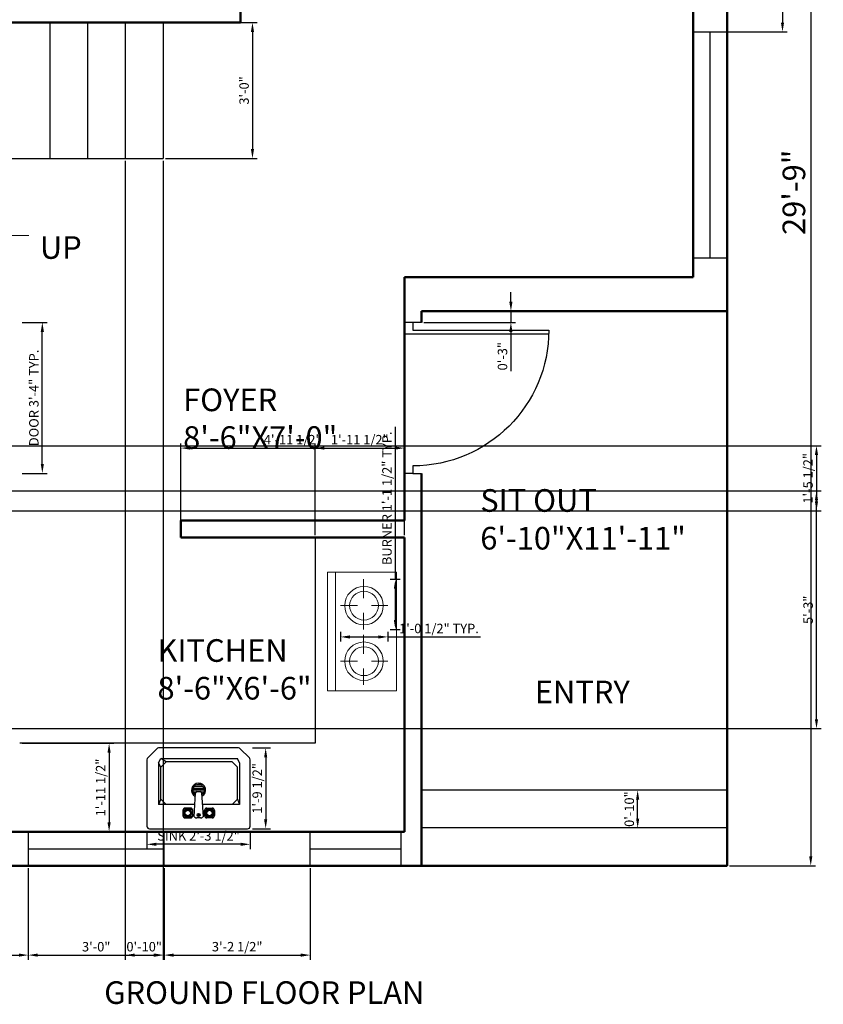
# Model space of a CAD drawing. Units: inches. Extents: x 3242 to 3618, y 1365 to 1814.
# Tile 3 of 6: x 3405 to 3618, y 1365 to 1626. Entities that reach past the tile are written whole.
import ezdxf

# ---------------------------------------------------------------- set-up
doc = ezdxf.new("R2010")
doc.units = ezdxf.units.IN
for name, color, linetype, lineweight in [('A-ANNO-DIMS', 2, 'Continuous', 18), ('A-ANNO-SYMB', 7, 'Continuous', 18), ('A-ANNO-TEXT', 7, 'Continuous', 25), ('A-AREA-IDEN', 7, 'Continuous', 25), ('A-DOOR', 4, 'Continuous', 25), ('A-EQPM', 8, 'Continuous', 18), ('A-FLOR-CASE', 8, 'Continuous', 25), ('A-FLOR-FIXT', 8, 'Continuous', 25), ('A-FLOR-STRS', 7, 'Continuous', 25), ('A-GLAZ', 5, 'Continuous', 25), ('A-WALL', 7, 'Continuous', 50)]:
    doc.layers.add(name, color=color, linetype=linetype, lineweight=lineweight)
doc.styles.get("Standard").update_dxf_attribs({"font": 'arial.ttf'})
doc.dimstyles.new('ISO-25', dxfattribs={"dimtxt": 2.5, "dimasz": 2.5, "dimexe": 1.25, "dimexo": 0.625, "dimtad": 1, "dimdec": 0, "dimlunit": 3, "dimtxsty": 'Standard', "dimcen": 2.5, "dimadec": 0, "dimazin": 0, "dimtfac": 1, "dimtdec": 0, "dimtmove": 0, "dimatfit": 3, "dimfxl": 1, "dimarcsym": 0})

# ---------------------------------------------------------------- blocks, each defined once
blk = doc.blocks.new('A$C4CB854FF')
for p, q in [((0.4725, 0.38), (0.0125, 0.38)), ((0, 0.3675), (0, 0.0552)), ((0.1787, 0.329), (0.2034, 0.329)), ((0.2337, 0.329), (0.2502, 0.329)), ((0.3052, 0.329), (0.2804, 0.329)), ((0.485, 0.0552), (0.485, 0.3675)), ((0.1677, 0.2932), (0.1677, 0.318)), ((0.1745, 0.2919), (0.1745, 0.3194)), ((0.1773, 0.3221), (0.2048, 0.3221)), ((0.2048, 0.2891), (0.1773, 0.2891)), ((0.2034, 0.2822), (0.1787, 0.2822)), ((0.2075, 0.3194), (0.2075, 0.2919)), ((0.2144, 0.318), (0.2144, 0.2932)), ((0.2279, 0.2104), (0.2213, 0.3235)), ((0.2625, 0.3235), (0.256, 0.2104)), ((0.2694, 0.318), (0.2694, 0.2932)), ((0.2763, 0.3194), (0.2763, 0.2919)), ((0.3065, 0.3221), (0.279, 0.3221)), ((0.279, 0.2891), (0.3065, 0.2891)), ((0.2804, 0.2822), (0.3052, 0.2822)), ((0.3093, 0.2919), (0.3093, 0.3194)), ((0.3162, 0.2932), (0.3162, 0.318)), ((0.05, 0.265), (0.2247, 0.265)), ((0.06, 0.24), (0.05, 0.265)), ((0.05, 0.07), (0.05, 0.265)), ((0.085, 0.265), (0.06, 0.24)), ((0.06, 0.24), (0.06, 0.09)), ((0.2591, 0.265), (0.43, 0.265)), ((0.395, 0.265), (0.42, 0.24)), ((0.42, 0.24), (0.43, 0.265)), ((0.42, 0.24), (0.42, 0.09)), ((0.43, 0.07), (0.43, 0.265)), ((0.2152, 0.1984), (0.2694, 0.1984)), ((0.2297, 0.2066), (0.2165, 0.2066)), ((0.2681, 0.1901), (0.2165, 0.1901)), ((0.2272, 0.2149), (0.2208, 0.2149)), ((0.2505, 0.2052), (0.2334, 0.2052)), ((0.2681, 0.2066), (0.2541, 0.2066)), ((0.2638, 0.2149), (0.2566, 0.2149)), ((0.2638, 0.1819), (0.2208, 0.1819)), ((0.2533, 0.1736), (0.2313, 0.1736)), ((0.0037, 0.0463), (0.0463, 0.0037)), ((0.05, 0.07), (0.06, 0.05)), ((0.06, 0.09), (0.085, 0.065)), ((0.42, 0.05), (0.06, 0.05)), ((0.085, 0.065), (0.395, 0.065)), ((0.42, 0.09), (0.395, 0.065)), ((0.395, 0.065), (0.42, 0.05)), ((0.42, 0.09), (0.43, 0.07)), ((0.43, 0.07), (0.42, 0.05)), ((0.4387, 0.0037), (0.4813, 0.0463)), ((0.0552, 0), (0.4298, 0))]:
    blk.add_line(p, q)
for centre, radius in [((0.191, 0.3056), 0.0165), ((0.191, 0.3056), 0.0127), ((0.2419, 0.3152), 0.00688), ((0.2419, 0.3152), 0.00344), ((0.2928, 0.3056), 0.0165), ((0.2928, 0.3056), 0.0127)]:
    blk.add_circle(centre, radius)
for centre, radius, start, end in [((0.0125, 0.3675), 0.0125, 90, 180), ((0.4725, 0.3675), 0.0125, 0, 90), ((0.1787, 0.318), 0.011, 90, 180), ((0.2034, 0.318), 0.011, 0, 90), ((0.2329, 0.314), 0.015, 87.1975, 140.7274), ((0.2509, 0.314), 0.015, 39.2726, 92.8025), ((0.2804, 0.318), 0.011, 90, 180), ((0.3052, 0.318), 0.011, 0, 90), ((0.1787, 0.2932), 0.011, 180, 270), ((0.1773, 0.3194), 0.00275, 90, 180), ((0.1773, 0.2919), 0.00275, 180, 270), ((0.2034, 0.2932), 0.011, 270, 0), ((0.2048, 0.3194), 0.00275, 360, 90), ((0.2048, 0.2919), 0.00275, 270, 0), ((0.2804, 0.2932), 0.011, 180, 270), ((0.279, 0.3194), 0.00275, 90, 180), ((0.279, 0.2919), 0.00275, 180, 270), ((0.3052, 0.2932), 0.011, 270, 360), ((0.3065, 0.3194), 0.00275, 360, 90), ((0.3065, 0.2919), 0.00275, 270, 0), ((0.2423, 0.1984), 0.033, 118.6883, 62.8686), ((0.2423, 0.1984), 0.0271, 124.7758, 57.2247), ((0.2334, 0.2107), 0.0055, 183.3274, 270), ((0.2505, 0.2107), 0.0055, 270, 356.6726), ((0.0125, 0.0552), 0.0125, 180, 225), ((0.4725, 0.0552), 0.0125, 315, 0), ((0.0552, 0.0125), 0.0125, 225, 270), ((0.4298, 0.0125), 0.0125, 270, 315)]:
    blk.add_arc(centre, radius, start, end)
blk = doc.blocks.new('*D4')
at = {"layer": 'A-ANNO-DIMS', "color": 0, "lineweight": -2, "transparency": 16777216}
for p, q in [((3593.11, 1758.66), (3615.91, 1758.66)), ((3614.66, 1756.16), (3614.66, 1404.16)), ((3593.11, 1401.66), (3615.91, 1401.66))]:
    blk.add_line(p, q, dxfattribs=at)
at = {"layer": 'A-ANNO-DIMS', "color": 0, "transparency": 16777216}
for points in [[(3614.24, 1756.16), (3615.08, 1756.16), (3614.66, 1758.66)], [(3614.24, 1404.16), (3615.08, 1404.16), (3614.66, 1401.66)]]:
    blk.add_solid(points, dxfattribs=at)
at = {"layer": 'Defpoints', "color": 0, "transparency": 16777216}
for p in [(3592.48, 1758.66), (3592.48, 1401.66), (3614.66, 1401.66)]:
    blk.add_point(p, dxfattribs=at)
at = {"layer": 'A-ANNO-DIMS', "color": 0, "transparency": 16777216, "insert": (3610.97, 1580.16), "char_height": 6, "attachment_point": 5, "rotation": 90}
blk.add_mtext('29\'-9"', dxfattribs=at)
blk = doc.blocks.new('DOOR-SWING-36IN')
for p, q in [((33.75, 40), (38.25, 40)), ((36, 40), (36, 38)), ((36, 38), (0, 38)), ((38.25, 37), (0, 37)), ((36, 0), (33.75, 0)), ((36, 2), (36, 0)), ((36, 0), (38.25, 0))]:
    blk.add_line(p, q)
blk.add_arc((36, 38), 36, 180, 270)
blk = doc.blocks.new('WINDOW-24IN')
for p, q in [((0, 9), (24, 9)), ((0, 0), (0, 9)), ((24, 9), (24, 0)), ((0, 4.5), (24, 4.5)), ((24, 0), (0, 0))]:
    blk.add_line(p, q)
blk = doc.blocks.new('WINDOW-60IN')
for p, q in [((0, 9), (60, 9)), ((0, 0), (0, 9)), ((60, 9), (60, 0)), ((0, 4.5), (60, 4.5)), ((60, 0), (0, 0))]:
    blk.add_line(p, q)
blk = doc.blocks.new('COOKTOP-BURNER')
at = {"ltscale": 120}
for p, q in [((6.09, 13.3), (6.09, 8.26)), ((0, 6.34), (4.54, 6.34)), ((8.26, 6.34), (12.57, 6.34)), ((6.09, 4.41), (6.09, 0))]:
    blk.add_line(p, q, dxfattribs=at)
for radius in [5.11, 3.82]:
    blk.add_circle((6.23, 6.3), radius, dxfattribs=at)
blk = doc.blocks.new('*D17')
at = {"layer": 'A-ANNO-DIMS', "color": 0, "lineweight": -2, "transparency": 16777216}
for p, q in [((3405.61, 1545.66), (3412.23, 1545.66)), ((3410.98, 1508.16), (3410.98, 1543.16)), ((3405.61, 1505.66), (3412.23, 1505.66))]:
    blk.add_line(p, q, dxfattribs=at)
at = {"layer": 'A-ANNO-DIMS', "color": 0, "transparency": 16777216}
for points in [[(3410.56, 1543.16), (3411.4, 1543.16), (3410.98, 1545.66)], [(3410.56, 1508.16), (3411.4, 1508.16), (3410.98, 1505.66)]]:
    blk.add_solid(points, dxfattribs=at)
at = {"layer": 'Defpoints', "color": 0, "transparency": 16777216}
for p in [(3404.98, 1545.66), (3410.98, 1545.66), (3404.98, 1505.66)]:
    blk.add_point(p, dxfattribs=at)
at = {"layer": 'A-ANNO-DIMS', "color": 0, "transparency": 16777216, "insert": (3409.06, 1525.66), "char_height": 2.5, "attachment_point": 5, "rotation": 90}
blk.add_mtext('DOOR 3\'-4" TYP.', dxfattribs=at)
blk = doc.blocks.new('*D25')
at = {"layer": 'A-ANNO-DIMS', "color": 0, "lineweight": -2, "transparency": 16777216}
for p, q in [((3438.7, 1410.81), (3438.7, 1406.08)), ((3466.07, 1410.81), (3466.07, 1406.08)), ((3463.57, 1407.33), (3441.2, 1407.33))]:
    blk.add_line(p, q, dxfattribs=at)
at = {"layer": 'A-ANNO-DIMS', "color": 0, "transparency": 16777216}
for points in [[(3441.2, 1407.75), (3441.2, 1406.91), (3438.7, 1407.33)], [(3463.57, 1407.75), (3463.57, 1406.91), (3466.07, 1407.33)]]:
    blk.add_solid(points, dxfattribs=at)
at = {"layer": 'Defpoints', "color": 0, "transparency": 16777216}
for p in [(3438.7, 1411.44), (3466.07, 1411.44), (3438.7, 1407.33)]:
    blk.add_point(p, dxfattribs=at)
at = {"layer": 'A-ANNO-DIMS', "color": 0, "transparency": 16777216, "insert": (3452.38, 1409.25), "char_height": 2.5, "attachment_point": 5}
blk.add_mtext('SINK 2\'-3 1/2"', dxfattribs=at)
blk = doc.blocks.new('*D26')
at = {"layer": 'A-ANNO-DIMS', "color": 0, "lineweight": -2, "transparency": 16777216}
for p, q in [((3466.69, 1432.88), (3471.43, 1432.88)), ((3470.18, 1430.38), (3470.18, 1413.94)), ((3466.69, 1411.44), (3471.43, 1411.44))]:
    blk.add_line(p, q, dxfattribs=at)
at = {"layer": 'A-ANNO-DIMS', "color": 0, "transparency": 16777216}
for points in [[(3469.76, 1430.38), (3470.59, 1430.38), (3470.18, 1432.88)], [(3469.76, 1413.94), (3470.59, 1413.94), (3470.18, 1411.44)]]:
    blk.add_solid(points, dxfattribs=at)
at = {"layer": 'Defpoints', "color": 0, "transparency": 16777216}
for p in [(3466.07, 1432.88), (3466.07, 1411.44), (3470.18, 1411.44)]:
    blk.add_point(p, dxfattribs=at)
at = {"layer": 'A-ANNO-DIMS', "color": 0, "transparency": 16777216, "insert": (3468.26, 1422.16), "char_height": 2.5, "attachment_point": 5, "rotation": 90}
blk.add_mtext('1\'-9 1/2"', dxfattribs=at)
blk = doc.blocks.new('*D27')
at = {"layer": 'A-ANNO-DIMS', "color": 0, "lineweight": -2, "transparency": 16777216}
for p, q in [((3504.57, 1477.59), (3504.57, 1518.01)), ((3503.2, 1477.59), (3505.82, 1477.59)), ((3504.57, 1466.79), (3504.57, 1475.09)), ((3503.2, 1464.29), (3505.82, 1464.29))]:
    blk.add_line(p, q, dxfattribs=at)
at = {"layer": 'A-ANNO-DIMS', "color": 0, "transparency": 16777216}
for points in [[(3504.15, 1475.09), (3504.99, 1475.09), (3504.57, 1477.59)], [(3504.15, 1466.79), (3504.99, 1466.79), (3504.57, 1464.29)]]:
    blk.add_solid(points, dxfattribs=at)
at = {"layer": 'Defpoints', "color": 0, "transparency": 16777216}
for p in [(3502.57, 1477.59), (3504.57, 1477.59), (3502.57, 1464.29)]:
    blk.add_point(p, dxfattribs=at)
at = {"layer": 'A-ANNO-DIMS', "color": 0, "transparency": 16777216, "insert": (3502.65, 1499.05), "char_height": 2.5, "attachment_point": 5, "rotation": 90}
blk.add_mtext('BURNER 1\'-1 1/2" TYP.', dxfattribs=at)
blk = doc.blocks.new('*D28')
at = {"layer": 'A-ANNO-DIMS', "color": 0, "lineweight": -2, "transparency": 16777216}
for p, q in [((3490.01, 1463.67), (3490.01, 1461.05)), ((3492.51, 1462.3), (3500.07, 1462.3)), ((3502.57, 1463.67), (3502.57, 1461.05)), ((3502.57, 1462.3), (3527.15, 1462.3))]:
    blk.add_line(p, q, dxfattribs=at)
at = {"layer": 'A-ANNO-DIMS', "color": 0, "transparency": 16777216}
for points in [[(3492.51, 1462.71), (3492.51, 1461.88), (3490.01, 1462.3)], [(3500.07, 1462.71), (3500.07, 1461.88), (3502.57, 1462.3)]]:
    blk.add_solid(points, dxfattribs=at)
at = {"layer": 'Defpoints', "color": 0, "transparency": 16777216}
for p in [(3490.01, 1464.29), (3502.57, 1464.29), (3502.57, 1462.3)]:
    blk.add_point(p, dxfattribs=at)
at = {"layer": 'A-ANNO-DIMS', "color": 0, "transparency": 16777216, "insert": (3516.11, 1464.22), "char_height": 2.5, "attachment_point": 5}
blk.add_mtext('1\'-0 1/2" TYP.', dxfattribs=at)
blk = doc.blocks.new('*D36')
at = {"layer": 'A-ANNO-DIMS', "color": 0, "lineweight": -2, "transparency": 16777216}
for p, q in [((3584.11, 1670.23), (3608.43, 1670.23)), ((3607.18, 1667.73), (3607.18, 1625.17)), ((3584.11, 1622.67), (3608.43, 1622.67))]:
    blk.add_line(p, q, dxfattribs=at)
at = {"layer": 'A-ANNO-DIMS', "color": 0, "transparency": 16777216}
for points in [[(3606.76, 1667.73), (3607.6, 1667.73), (3607.18, 1670.23)], [(3606.76, 1625.17), (3607.6, 1625.17), (3607.18, 1622.67)]]:
    blk.add_solid(points, dxfattribs=at)
at = {"layer": 'Defpoints', "color": 0, "transparency": 16777216}
for p in [(3583.48, 1670.23), (3583.48, 1622.67), (3607.18, 1622.67)]:
    blk.add_point(p, dxfattribs=at)
at = {"layer": 'A-ANNO-DIMS', "color": 0, "transparency": 16777216, "insert": (3605.26, 1646.45), "char_height": 2.5, "attachment_point": 5, "rotation": 90}
blk.add_mtext('3\'-11 1/2"', dxfattribs=at)
blk = doc.blocks.new('*D40')
at = {"layer": 'A-ANNO-DIMS', "color": 0, "lineweight": -2, "transparency": 16777216}
for p, q in [((3375.35, 1401.03), (3375.35, 1376.71)), ((3407.26, 1401.03), (3407.26, 1376.71)), ((3377.85, 1377.96), (3404.76, 1377.96))]:
    blk.add_line(p, q, dxfattribs=at)
at = {"layer": 'A-ANNO-DIMS', "color": 0, "transparency": 16777216}
for points in [[(3377.85, 1378.37), (3377.85, 1377.54), (3375.35, 1377.96)], [(3404.76, 1378.37), (3404.76, 1377.54), (3407.26, 1377.96)]]:
    blk.add_solid(points, dxfattribs=at)
at = {"layer": 'Defpoints', "color": 0, "transparency": 16777216}
for p in [(3375.35, 1401.66), (3407.26, 1401.66), (3407.26, 1377.96)]:
    blk.add_point(p, dxfattribs=at)
at = {"layer": 'A-ANNO-DIMS', "color": 0, "transparency": 16777216, "insert": (3391.3, 1379.86), "char_height": 2.5, "attachment_point": 5}
blk.add_mtext('2\'-8"', dxfattribs=at)
blk = doc.blocks.new('*D41')
at = {"layer": 'A-ANNO-DIMS', "color": 0, "lineweight": -2, "transparency": 16777216}
for p, q in [((3407.26, 1401.03), (3407.26, 1376.71)), ((3443.26, 1401.03), (3443.26, 1376.71)), ((3409.76, 1377.96), (3440.76, 1377.96))]:
    blk.add_line(p, q, dxfattribs=at)
at = {"layer": 'A-ANNO-DIMS', "color": 0, "transparency": 16777216}
for points in [[(3409.76, 1378.37), (3409.76, 1377.54), (3407.26, 1377.96)], [(3440.76, 1378.37), (3440.76, 1377.54), (3443.26, 1377.96)]]:
    blk.add_solid(points, dxfattribs=at)
at = {"layer": 'Defpoints', "color": 0, "transparency": 16777216}
for p in [(3407.26, 1401.66), (3443.26, 1401.66), (3443.26, 1377.96)]:
    blk.add_point(p, dxfattribs=at)
at = {"layer": 'A-ANNO-DIMS', "color": 0, "transparency": 16777216, "insert": (3425.26, 1379.86), "char_height": 2.5, "attachment_point": 5}
blk.add_mtext('3\'-0"', dxfattribs=at)
blk = doc.blocks.new('*D42')
at = {"layer": 'A-ANNO-DIMS', "color": 0, "lineweight": -2, "transparency": 16777216}
for p, q in [((3443.26, 1401.03), (3443.26, 1376.71)), ((3482, 1401.03), (3482, 1376.71)), ((3445.76, 1377.96), (3479.5, 1377.96))]:
    blk.add_line(p, q, dxfattribs=at)
at = {"layer": 'A-ANNO-DIMS', "color": 0, "transparency": 16777216}
for points in [[(3445.76, 1378.37), (3445.76, 1377.54), (3443.26, 1377.96)], [(3479.5, 1378.37), (3479.5, 1377.54), (3482, 1377.96)]]:
    blk.add_solid(points, dxfattribs=at)
at = {"layer": 'Defpoints', "color": 0, "transparency": 16777216}
for p in [(3443.26, 1401.66), (3482, 1401.66), (3482, 1377.96)]:
    blk.add_point(p, dxfattribs=at)
at = {"layer": 'A-ANNO-DIMS', "color": 0, "transparency": 16777216, "insert": (3462.63, 1379.87), "char_height": 2.5, "attachment_point": 5}
blk.add_mtext('3\'-2 1/2"', dxfattribs=at)
blk = doc.blocks.new('*D43')
at = {"layer": 'A-ANNO-DIMS', "color": 0, "lineweight": -2, "transparency": 16777216}
for p, q in [((3432.98, 1588.53), (3432.98, 1376.71)), ((3442.98, 1588.53), (3442.98, 1376.71)), ((3435.48, 1377.96), (3440.48, 1377.96))]:
    blk.add_line(p, q, dxfattribs=at)
at = {"layer": 'A-ANNO-DIMS', "color": 0, "transparency": 16777216}
for points in [[(3435.48, 1378.37), (3435.48, 1377.54), (3432.98, 1377.96)], [(3440.48, 1378.37), (3440.48, 1377.54), (3442.98, 1377.96)]]:
    blk.add_solid(points, dxfattribs=at)
at = {"layer": 'Defpoints', "color": 0, "transparency": 16777216}
for p in [(3432.98, 1589.16), (3442.98, 1589.16), (3442.98, 1377.96)]:
    blk.add_point(p, dxfattribs=at)
at = {"layer": 'A-ANNO-DIMS', "color": 0, "transparency": 16777216, "insert": (3437.98, 1379.86), "char_height": 2.5, "attachment_point": 5}
blk.add_mtext('0\'-10"', dxfattribs=at)
blk = doc.blocks.new('*D44')
at = {"layer": 'A-ANNO-DIMS', "color": 0, "lineweight": -2, "transparency": 16777216}
for p, q in [((3443.61, 1625.16), (3467.93, 1625.16)), ((3466.68, 1622.66), (3466.68, 1591.66)), ((3443.61, 1589.16), (3467.93, 1589.16))]:
    blk.add_line(p, q, dxfattribs=at)
at = {"layer": 'A-ANNO-DIMS', "color": 0, "transparency": 16777216}
for points in [[(3466.26, 1622.66), (3467.1, 1622.66), (3466.68, 1625.16)], [(3466.26, 1591.66), (3467.1, 1591.66), (3466.68, 1589.16)]]:
    blk.add_solid(points, dxfattribs=at)
at = {"layer": 'Defpoints', "color": 0, "transparency": 16777216}
for p in [(3442.98, 1625.16), (3442.98, 1589.16), (3466.68, 1589.16)]:
    blk.add_point(p, dxfattribs=at)
at = {"layer": 'A-ANNO-DIMS', "color": 0, "transparency": 16777216, "insert": (3464.78, 1607.16), "char_height": 2.5, "attachment_point": 5, "rotation": 90}
blk.add_mtext('3\'-0"', dxfattribs=at)
blk = doc.blocks.new('*D45')
at = {"layer": 'A-ANNO-DIMS', "color": 0, "lineweight": -2, "transparency": 16777216}
for p, q in [((3405.61, 1434.12), (3429.93, 1434.12)), ((3428.68, 1431.62), (3428.68, 1413.16)), ((3405.61, 1410.66), (3429.93, 1410.66))]:
    blk.add_line(p, q, dxfattribs=at)
at = {"layer": 'A-ANNO-DIMS', "color": 0, "transparency": 16777216}
for points in [[(3428.26, 1431.62), (3429.1, 1431.62), (3428.68, 1434.12)], [(3428.26, 1413.16), (3429.1, 1413.16), (3428.68, 1410.66)]]:
    blk.add_solid(points, dxfattribs=at)
at = {"layer": 'Defpoints', "color": 0, "transparency": 16777216}
for p in [(3404.98, 1434.12), (3404.98, 1410.66), (3428.68, 1410.66)]:
    blk.add_point(p, dxfattribs=at)
at = {"layer": 'A-ANNO-DIMS', "color": 0, "transparency": 16777216, "insert": (3426.76, 1422.39), "char_height": 2.5, "attachment_point": 5, "rotation": 90}
blk.add_mtext('1\'-11 1/2"', dxfattribs=at)
blk = doc.blocks.new('*D46')
at = {"layer": 'A-ANNO-DIMS', "color": 0, "lineweight": -2, "transparency": 16777216}
for p, q in [((3483.26, 1489.28), (3483.26, 1513.61)), ((3485.76, 1512.36), (3504.48, 1512.36)), ((3506.98, 1489.28), (3506.98, 1513.61))]:
    blk.add_line(p, q, dxfattribs=at)
at = {"layer": 'A-ANNO-DIMS', "color": 0, "transparency": 16777216}
for points in [[(3485.76, 1512.77), (3485.76, 1511.94), (3483.26, 1512.36)], [(3504.48, 1512.77), (3504.48, 1511.94), (3506.98, 1512.36)]]:
    blk.add_solid(points, dxfattribs=at)
at = {"layer": 'Defpoints', "color": 0, "transparency": 16777216}
for p in [(3506.98, 1512.36), (3483.26, 1488.66), (3506.98, 1488.66)]:
    blk.add_point(p, dxfattribs=at)
at = {"layer": 'A-ANNO-DIMS', "color": 0, "transparency": 16777216, "insert": (3495.12, 1514.27), "char_height": 2.5, "attachment_point": 5}
blk.add_mtext('1\'-11 1/2"', dxfattribs=at)
blk = doc.blocks.new('*D54')
at = {"layer": 'A-ANNO-DIMS', "color": 0, "lineweight": -2, "transparency": 16777216}
for p, q in [((3362.21, 1500.99), (3617.43, 1500.99)), ((3616.18, 1440.49), (3616.18, 1498.49)), ((3362.21, 1437.99), (3617.43, 1437.99))]:
    blk.add_line(p, q, dxfattribs=at)
at = {"layer": 'A-ANNO-DIMS', "color": 0, "transparency": 16777216}
for points in [[(3615.76, 1498.49), (3616.6, 1498.49), (3616.18, 1500.99)], [(3615.76, 1440.49), (3616.6, 1440.49), (3616.18, 1437.99)]]:
    blk.add_solid(points, dxfattribs=at)
at = {"layer": 'Defpoints', "color": 0, "transparency": 16777216}
for p in [(3361.59, 1500.99), (3616.18, 1500.99), (3361.59, 1437.99)]:
    blk.add_point(p, dxfattribs=at)
at = {"layer": 'A-ANNO-DIMS', "color": 0, "transparency": 16777216, "insert": (3614.28, 1469.49), "char_height": 2.5, "attachment_point": 5, "rotation": 90}
blk.add_mtext('5\'-3"', dxfattribs=at)
blk = doc.blocks.new('*D55')
at = {"layer": 'A-ANNO-DIMS', "color": 0, "lineweight": -2, "transparency": 16777216}
for p, q in [((3303.13, 1513), (3617.43, 1513)), ((3616.18, 1510.5), (3616.18, 1498.21)), ((3303.13, 1495.71), (3617.43, 1495.71))]:
    blk.add_line(p, q, dxfattribs=at)
at = {"layer": 'A-ANNO-DIMS', "color": 0, "transparency": 16777216}
for points in [[(3615.76, 1510.5), (3616.6, 1510.5), (3616.18, 1513)], [(3615.76, 1498.21), (3616.6, 1498.21), (3616.18, 1495.71)]]:
    blk.add_solid(points, dxfattribs=at)
at = {"layer": 'Defpoints', "color": 0, "transparency": 16777216}
for p in [(3302.5, 1513), (3302.5, 1495.71), (3616.18, 1495.71)]:
    blk.add_point(p, dxfattribs=at)
at = {"layer": 'A-ANNO-DIMS', "color": 0, "transparency": 16777216, "insert": (3614.26, 1504.35), "char_height": 2.5, "attachment_point": 5, "rotation": 90}
blk.add_mtext('1\'-5 1/2"', dxfattribs=at)
blk = doc.blocks.new('*D61')
at = {"layer": 'A-ANNO-DIMS', "color": 0, "lineweight": -2, "transparency": 16777216}
for p, q in [((3591.86, 1421.66), (3567.53, 1421.66)), ((3568.78, 1414.16), (3568.78, 1419.16)), ((3591.86, 1411.66), (3567.53, 1411.66))]:
    blk.add_line(p, q, dxfattribs=at)
at = {"layer": 'A-ANNO-DIMS', "color": 0, "transparency": 16777216}
for points in [[(3568.36, 1419.16), (3569.2, 1419.16), (3568.78, 1421.66)], [(3568.36, 1414.16), (3569.2, 1414.16), (3568.78, 1411.66)]]:
    blk.add_solid(points, dxfattribs=at)
at = {"layer": 'Defpoints', "color": 0, "transparency": 16777216}
for p in [(3568.78, 1421.66), (3592.48, 1421.66), (3592.48, 1411.66)]:
    blk.add_point(p, dxfattribs=at)
at = {"layer": 'A-ANNO-DIMS', "color": 0, "transparency": 16777216, "insert": (3566.88, 1416.66), "char_height": 2.5, "attachment_point": 5, "rotation": 90}
blk.add_mtext('0\'-10"', dxfattribs=at)
blk = doc.blocks.new('*D62')
at = {"layer": 'A-ANNO-DIMS', "color": 0, "lineweight": -2, "transparency": 16777216}
for p, q in [((3535.18, 1551.16), (3535.18, 1553.66)), ((3512.11, 1548.66), (3536.43, 1548.66)), ((3535.18, 1548.66), (3535.18, 1545.66)), ((3512.11, 1545.66), (3536.43, 1545.66)), ((3535.18, 1543.16), (3535.18, 1532.76))]:
    blk.add_line(p, q, dxfattribs=at)
at = {"layer": 'A-ANNO-DIMS', "color": 0, "transparency": 16777216}
for points in [[(3534.76, 1551.16), (3535.6, 1551.16), (3535.18, 1548.66)], [(3534.76, 1543.16), (3535.6, 1543.16), (3535.18, 1545.66)]]:
    blk.add_solid(points, dxfattribs=at)
at = {"layer": 'Defpoints', "color": 0, "transparency": 16777216}
for p in [(3511.48, 1548.66), (3511.48, 1545.66), (3535.18, 1545.66)]:
    blk.add_point(p, dxfattribs=at)
at = {"layer": 'A-ANNO-DIMS', "color": 0, "transparency": 16777216, "insert": (3533.28, 1536.71), "char_height": 2.5, "attachment_point": 5, "rotation": 90}
blk.add_mtext('0\'-3"', dxfattribs=at)
blk = doc.blocks.new('*D63')
at = {"layer": 'A-ANNO-DIMS', "color": 0, "lineweight": -2, "transparency": 16777216}
for p, q in [((3447.7, 1489.28), (3447.7, 1513.61)), ((3450.2, 1512.36), (3504.48, 1512.36)), ((3506.98, 1489.28), (3506.98, 1513.61))]:
    blk.add_line(p, q, dxfattribs=at)
at = {"layer": 'A-ANNO-DIMS', "color": 0, "transparency": 16777216}
for points in [[(3450.2, 1512.77), (3450.2, 1511.94), (3447.7, 1512.36)], [(3504.48, 1512.77), (3504.48, 1511.94), (3506.98, 1512.36)]]:
    blk.add_solid(points, dxfattribs=at)
at = {"layer": 'Defpoints', "color": 0, "transparency": 16777216}
for p in [(3506.98, 1512.36), (3447.7, 1488.66), (3506.98, 1488.66)]:
    blk.add_point(p, dxfattribs=at)
at = {"layer": 'A-ANNO-DIMS', "color": 0, "transparency": 16777216, "insert": (3477.34, 1514.27), "char_height": 2.5, "attachment_point": 5}
blk.add_mtext('4\'-11 1/2"', dxfattribs=at)

msp = doc.modelspace()

# ---------------------------------------------------------------- linework, layer by layer
at = {"layer": 'A-ANNO-SYMB'}
msp.add_line((3407.4, 1568.69), (3336.54, 1568.69), dxfattribs=at)
at = {"layer": 'A-EQPM', "ltscale": 120}
for p, q in [((3486.53, 1479.45), (3486.53, 1448.02)), ((3504.89, 1479.45), (3486.53, 1479.45)), ((3488.69, 1479.45), (3488.69, 1448.02)), ((3504.89, 1448.02), (3504.89, 1479.45)), ((3486.53, 1448.02), (3504.89, 1448.02))]:
    msp.add_line(p, q, dxfattribs=at)
at = {"layer": 'A-FLOR-CASE'}
for p, q in [((3483.26, 1488.66), (3483.26, 1434.12)), ((3483.26, 1434.12), (3404.98, 1434.12))]:
    msp.add_line(p, q, dxfattribs=at)
at = {"layer": 'A-FLOR-STRS'}
for p, q in [((3412.98, 1625.16), (3412.98, 1589.16)), ((3422.98, 1625.16), (3422.98, 1589.16)), ((3432.98, 1625.16), (3432.98, 1589.16)), ((3442.98, 1625.16), (3442.98, 1589.16)), ((3332.98, 1589.16), (3442.98, 1589.16)), ((3592.48, 1421.66), (3511.48, 1421.66)), ((3592.48, 1411.66), (3511.48, 1411.66))]:
    msp.add_line(p, q, dxfattribs=at)
at = {"layer": 'A-GLAZ'}
for p, q in [((3443.26, 1410.66), (3407.26, 1410.66)), ((3407.26, 1410.66), (3407.26, 1401.66)), ((3443.26, 1401.66), (3443.26, 1410.66)), ((3407.26, 1406.16), (3443.26, 1406.16)), ((3407.26, 1401.66), (3443.26, 1401.66))]:
    msp.add_line(p, q, dxfattribs=at)
at = {"layer": 'A-WALL'}
for p, q in [((3592.48, 1758.66), (3592.48, 1401.66)), ((3463.48, 1749.66), (3463.48, 1625.16)), ((3583.48, 1749.66), (3583.48, 1557.66)), ((3280.48, 1625.16), (3463.48, 1625.16)), ((3506.98, 1553.16), (3506.98, 1557.66)), ((3506.98, 1557.66), (3511.48, 1557.66)), ((3511.48, 1557.66), (3583.48, 1557.66)), ((3506.98, 1553.16), (3506.98, 1493.16)), ((3511.48, 1548.66), (3511.48, 1545.66)), ((3511.48, 1548.66), (3583.48, 1548.66)), ((3583.48, 1548.66), (3592.48, 1548.66)), ((3511.48, 1505.66), (3511.48, 1410.66)), ((3447.7, 1493.16), (3506.98, 1493.16)), ((3447.7, 1493.16), (3447.7, 1488.66)), ((3447.7, 1488.66), (3506.98, 1488.66)), ((3506.98, 1488.66), (3506.98, 1410.66)), ((3280.48, 1410.66), (3506.98, 1410.66)), ((3511.48, 1410.66), (3511.48, 1401.66)), ((3271.48, 1401.66), (3592.48, 1401.66))]:
    msp.add_line(p, q, dxfattribs=at)

# ---------------------------------------------------------------- block references
at = {"layer": 'A-DOOR', "extrusion": (0, 0, -1), "zscale": -1}
msp.add_blockref('DOOR-SWING-36IN', (-3545.23, 1505.65), dxfattribs=at)
at = {"layer": 'A-EQPM'}
for p in [(3490.01, 1464.29), (3490.01, 1449.56)]:
    msp.add_blockref('COOKTOP-BURNER', p, dxfattribs=at)
at = {"layer": 'A-FLOR-FIXT', "xscale": 56.43950728980954, "yscale": 56.43950728980954, "zscale": 56.43950728980954, "rotation": 180}
msp.add_blockref('A$C4CB854FF', (3466.07, 1432.88), dxfattribs=at)
at = {"layer": 'A-GLAZ', "rotation": 89.99999999999946}
msp.add_blockref('WINDOW-60IN', (3592.48, 1562.67), dxfattribs=at)
at = {"layer": 'A-GLAZ'}
msp.add_blockref('WINDOW-24IN', (3482, 1401.65), dxfattribs=at)

# ---------------------------------------------------------------- texts
at = {"layer": 'A-ANNO-TEXT', "char_height": 6, "attachment_point": 1}
for s, insert in [('UP', (3410.34, 1568.53)), ('GROUND FLOOR PLAN', (3427.38, 1371.02))]:
    msp.add_mtext(s, dxfattribs=dict(at, insert=insert))
at = {"layer": 'A-ANNO-TEXT', "insert": (3541.52, 1450.72), "char_height": 6, "attachment_point": 1}
msp.add_mtext_dynamic_manual_height_columns('ENTRY', width=4.1892, gutter_width=12.5, heights=[0], dxfattribs=at)
at = {"layer": 'A-AREA-IDEN', "char_height": 6, "attachment_point": 1}
for s, insert in [('FOYER\\P8\'-6"X7\'-0"', (3448.31, 1528.15)), ('SIT OUT\\P6\'-10"X11\'-11"', (3527.07, 1501.47)), ('KITCHEN\\P8\'-6"X6\'-6"', (3441.5, 1461.7))]:
    msp.add_mtext(s, dxfattribs=dict(at, insert=insert))

# ---------------------------------------------------------------- dimensions: what is measured, and where the dimension line sits
at = {"layer": 'A-ANNO-DIMS'}
for base, p1, p2, angle, override, picture, middle in [((3614.66, 1401.66), (3592.48, 1758.66), (3592.48, 1401.66), 90, {"dimtxt": 6, "dimclrd": 0, "dimclre": 0, "dimclrt": 0}, '*D4', (3610.97, 1580.16)), ((3607.18, 1622.67), (3583.48, 1670.23), (3583.48, 1622.67), 270, {"dimdec": 1, "dimlfac": 1, "dimrnd": 0, "dimzin": 1, "dimdsep": 46, "dimlunit": 4, "dimfrac": 2}, '*D36', (3605.26, 1646.45)), ((3466.68, 1589.16), (3442.98, 1625.16), (3442.98, 1589.16), 270, {"dimdec": 1, "dimlfac": 1, "dimrnd": 0, "dimzin": 1, "dimdsep": 46, "dimlunit": 4, "dimfrac": 2}, '*D44', (3464.78, 1607.16)), ((3535.18, 1545.66), (3511.48, 1548.66), (3511.48, 1545.66), 270, {"dimdec": 1, "dimlfac": 1, "dimrnd": 0, "dimzin": 1, "dimdsep": 46, "dimlunit": 4, "dimfrac": 2}, '*D62', (3533.28, 1536.71)), ((3616.18, 1495.71), (3302.5, 1513), (3302.5, 1495.71), 90, {"dimdec": 1, "dimlfac": 1, "dimrnd": 0, "dimzin": 1, "dimdsep": 46, "dimlunit": 4, "dimfrac": 2}, '*D55', (3614.26, 1504.35)), ((3616.18, 1500.99), (3361.59, 1437.99), (3361.59, 1500.99), 90, {"dimdec": 1, "dimlfac": 1, "dimrnd": 0, "dimzin": 1, "dimdsep": 46, "dimlunit": 4, "dimfrac": 2}, '*D54', (3614.28, 1469.49)), ((3428.68, 1410.66), (3404.98, 1434.12), (3404.98, 1410.66), 270, {"dimdec": 1, "dimlfac": 1, "dimrnd": 0, "dimzin": 1, "dimdsep": 46, "dimlunit": 4, "dimfrac": 2}, '*D45', (3426.76, 1422.39)), ((3470.18, 1411.44), (3466.07, 1432.88), (3466.07, 1411.44), 270, {"dimdec": 1, "dimlfac": 1, "dimrnd": 0, "dimzin": 1, "dimdsep": 46, "dimlunit": 4, "dimfrac": 2}, '*D26', (3468.26, 1422.16)), ((3568.78, 1421.66), (3592.48, 1411.66), (3592.48, 1421.66), 90, {"dimdec": 1, "dimlfac": 1, "dimrnd": 0, "dimzin": 1, "dimdsep": 46, "dimlunit": 4, "dimfrac": 2}, '*D61', (3566.88, 1416.66))]:
    dim = msp.add_linear_dim(base=base, p1=p1, p2=p2, angle=angle, dimstyle='ISO-25', override=override, dxfattribs=at)
    dim.commit()
    dim.dimension.update_dxf_attribs({"geometry": picture, "text_midpoint": middle})
for base, p1, p2, picture, middle in [((3442.98, 1377.96), (3432.98, 1589.16), (3442.98, 1589.16), '*D43', (3437.98, 1379.86)), ((3506.98, 1512.36), (3447.7, 1488.66), (3506.98, 1488.66), '*D63', (3477.34, 1514.27)), ((3506.98, 1512.36), (3483.26, 1488.66), (3506.98, 1488.66), '*D46', (3495.12, 1514.27)), ((3407.26, 1377.96), (3375.35, 1401.66), (3407.26, 1401.66), '*D40', (3391.3, 1379.86)), ((3443.26, 1377.96), (3407.26, 1401.66), (3443.26, 1401.66), '*D41', (3425.26, 1379.86)), ((3482, 1377.96), (3443.26, 1401.66), (3482, 1401.66), '*D42', (3462.63, 1379.87))]:
    dim = msp.add_linear_dim(base=base, p1=p1, p2=p2, dimstyle='ISO-25', override={"dimdec": 1, "dimlfac": 1, "dimrnd": 0, "dimzin": 1, "dimdsep": 46, "dimlunit": 4, "dimfrac": 2}, dxfattribs=at)
    dim.commit()
    dim.dimension.update_dxf_attribs({"geometry": picture, "text_midpoint": middle})
for base, p1, p2, angle, text, picture, middle in [((3410.98, 1545.66), (3404.98, 1505.66), (3404.98, 1545.66), 90, 'DOOR <> TYP.', '*D17', (3409.06, 1525.66)), ((3504.57, 1477.59), (3502.57, 1464.29), (3502.57, 1477.59), 90, 'BURNER <> TYP.', '*D27', (3502.65, 1499.05)), ((3438.7, 1407.33), (3466.07, 1411.44), (3438.7, 1411.44), 180, 'SINK <>', '*D25', (3452.38, 1409.25))]:
    dim = msp.add_linear_dim(base=base, p1=p1, p2=p2, angle=angle, text=text, dimstyle='ISO-25', override={"dimdec": 1, "dimlfac": 1, "dimrnd": 0, "dimzin": 1, "dimdsep": 46, "dimlunit": 4, "dimfrac": 2}, dxfattribs=at)
    dim.commit()
    dim.dimension.update_dxf_attribs({"geometry": picture, "text_midpoint": middle})
dim = msp.add_linear_dim(base=(3502.57, 1462.3), p1=(3490.01, 1464.29), p2=(3502.57, 1464.29), text='<> TYP.', dimstyle='ISO-25', override={"dimdec": 1, "dimlfac": 1, "dimrnd": 0, "dimzin": 1, "dimdsep": 46, "dimlunit": 4, "dimfrac": 2}, dxfattribs=at)
dim.commit()
dim.dimension.update_dxf_attribs({"geometry": '*D28', "text_midpoint": (3516.11, 1464.22)})

doc.saveas('drawing.dxf')
